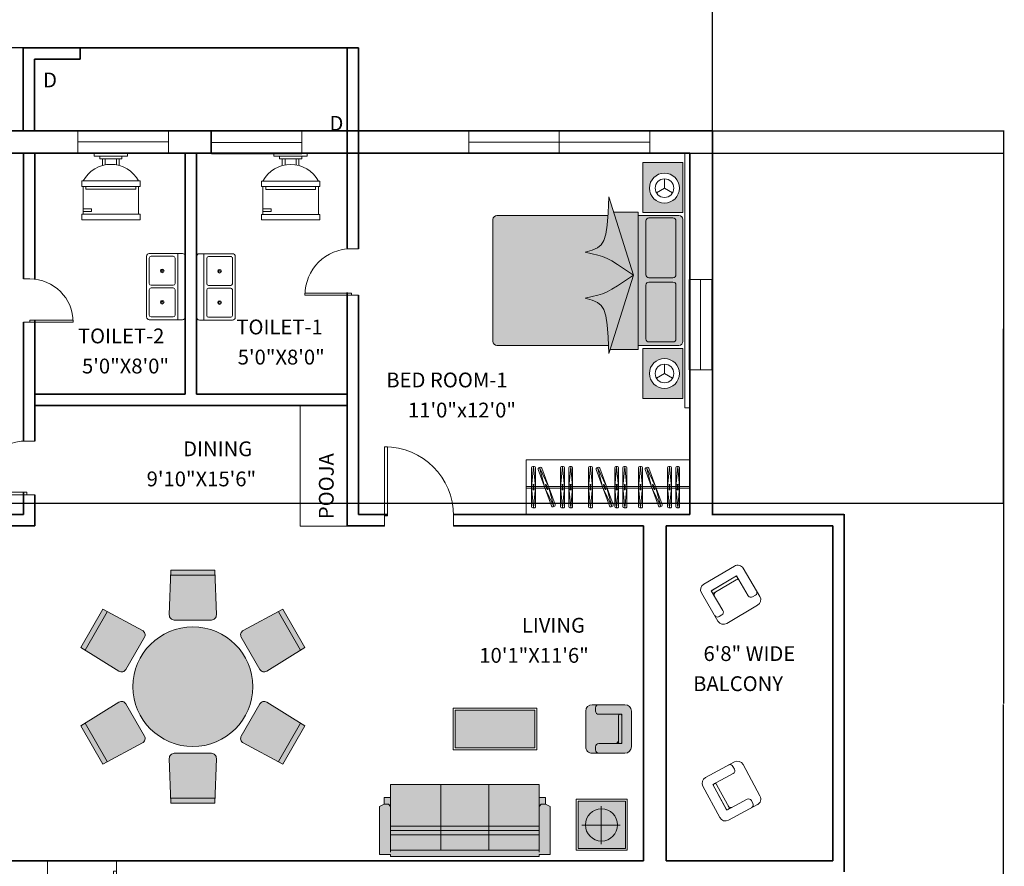
# Model space of a CAD drawing. Units: millimetres. Extents: x 27017497 to 27018854, y 7058029 to 7059154.
# Tile 90 of 91: x 27018462 to 27018854, y 7058297 to 7058634. Entities that reach past the tile are written whole.
import ezdxf

# ---------------------------------------------------------------- set-up
doc = ezdxf.new("R2010")
doc.units = ezdxf.units.MM
for name, color, linetype, lineweight in [('A-ANNO-DIMS', 2, 'Continuous', 18), ('A-ANNO-IDEN', 7, 'Continuous', 18), ('A-AREA-IDEN', 7, 'Continuous', 18), ('A-DOOR', 4, 'Continuous', 20), ('A-FLOR-CASE', 8, 'Continuous', 20), ('A-FLOR-FIXT', 9, 'Continuous', 18), ('A-FURN', 8, 'Continuous', 18), ('A-GLAZ', 4, 'Continuous', 18), ('A-WALL', 7, 'Continuous', 35)]:
    doc.layers.add(name, color=color, linetype=linetype, lineweight=lineweight)
doc.layers.add('A-FURN-PATT', color=177, linetype='Continuous', lineweight=13, true_color=0x293189)
doc.styles.get("Standard").update_dxf_attribs({"font": 'arial.ttf'})
doc.dimstyles.get("Standard").update_dxf_attribs({"dimtxt": 0.18, "dimasz": 0.18, "dimexe": 0.18, "dimexo": 0.0625, "dimgap": 0.09, "dimtad": 0, "dimtih": 1, "dimtoh": 1, "dimdec": 4, "dimzin": 0, "dimdsep": 46, "dimtxsty": 'Standard', "dimcen": 0.09, "dimadec": 0, "dimazin": 0, "dimtfac": 1, "dimtdec": 4, "dimtofl": 0, "dimtmove": 0, "dimatfit": 3, "dimfxl": 1, "dimtolj": 1, "dimtzin": 0, "dimarcsym": 0})

# ---------------------------------------------------------------- blocks, each defined once
blk = doc.blocks.new('CAMMAT')
for p, q in [((1.2731, 0), (-1.2731, 0)), ((1.2731, 0), (1.2731, -0.05)), ((-1.2731, 0), (-1.2731, -0.05)), ((1.2731, -0.05), (-1.2731, -0.05)), ((-1.18, -0.07), (-1.18, -0.47)), ((-1.18, -0.07), (-0.68, -0.07)), ((-0.68, -0.07), (-0.68, -0.47)), ((0.61, -0.07), (-0.61, -0.07)), ((0.68, -0.07), (0.68, -0.47)), ((0.68, -0.07), (1.18, -0.07)), ((1.18, -0.07), (1.18, -0.47)), ((-0.931, -0.2541), (-0.9775, -0.1737)), ((-0.65, -0.11), (-0.65, -0.5169)), ((-0.6152, -0.1695), (-0.6152, -0.4095)), ((-0.0465, -0.1395), (-0.5852, -0.1395)), ((-0.0165, -0.1695), (-0.0165, -0.4095)), ((0.0274, -0.1695), (0.0274, -0.4095)), ((0.5962, -0.1395), (0.0574, -0.1395)), ((0.6262, -0.1695), (0.6262, -0.4095)), ((0.65, -0.11), (0.65, -0.5169)), ((0.9242, -0.2541), (0.8777, -0.1737)), ((-0.931, -0.2541), (-0.9775, -0.3346)), ((-0.931, -0.2541), (-0.8381, -0.2541)), ((0.9242, -0.2541), (0.8777, -0.3346)), ((0.9242, -0.2541), (1.0171, -0.2541)), ((-1.18, -0.47), (-0.68, -0.47)), ((-0.0465, -0.4395), (-0.5852, -0.4395)), ((0.5962, -0.4395), (0.0574, -0.4395)), ((0.68, -0.47), (1.18, -0.47)), ((0.0535, -0.5623), (-0.7312, -0.8093)), ((-0.6904, -0.5169), (-0.6904, -0.8)), ((-0.6904, -0.5169), (0.6826, -0.5169)), ((0.0535, -0.5623), (0.8382, -0.8093)), ((0.6826, -0.5169), (0.6826, -0.7603)), ((-0.65, -0.8139), (-0.65, -1.93)), ((0.65, -0.8204), (0.65, -1.93)), ((0.61, -1.97), (-0.61, -1.97))]:
    blk.add_line(p, q)
for points in [[(-0.1761, -1.0476), (-0.161, -0.9772), (-0.1474, -0.921), (-0.1326, -0.8732), (-0.1139, -0.8282), (-0.0886, -0.7803), (-0.0541, -0.7238), (-0.0076, -0.653), (0.0535, -0.5623)], [(0.2832, -1.0476), (0.2681, -0.9772), (0.2545, -0.921), (0.2396, -0.8732), (0.2209, -0.8282), (0.1957, -0.7803), (0.1611, -0.7238), (0.1147, -0.653), (0.0535, -0.5623)], [(-0.7312, -0.8093), (-0.5683, -0.8185), (-0.4451, -0.828), (-0.3552, -0.8406), (-0.2919, -0.8591), (-0.2489, -0.8862), (-0.2196, -0.9248), (-0.1975, -0.9777), (-0.1761, -1.0476)], [(0.8382, -0.8093), (0.6753, -0.8185), (0.5522, -0.828), (0.4622, -0.8406), (0.399, -0.8591), (0.356, -0.8862), (0.3267, -0.9248), (0.3046, -0.9777), (0.2832, -1.0476)]]:
    blk.add_lwpolyline(points)
for centre, radius in [((-0.931, -0.2541), 0.15), ((-0.931, -0.2541), 0.0929), ((0.9242, -0.2541), 0.15), ((0.9242, -0.2541), 0.0929)]:
    blk.add_circle(centre, radius)
for centre, radius, start, end in [((-0.61, -0.11), 0.04, 90, 180), ((0.61, -0.11), 0.04, 0, 90), ((-0.5852, -0.1695), 0.03, 90, 180), ((-0.0465, -0.1695), 0.03, 360, 90), ((0.0574, -0.1695), 0.03, 90, 180), ((0.5962, -0.1695), 0.03, 360, 90), ((-0.5852, -0.4095), 0.03, 180, 270), ((-0.0465, -0.4095), 0.03, 270, 360), ((0.0574, -0.4095), 0.03, 180, 270), ((0.5962, -0.4095), 0.03, 270, 360), ((-0.61, -1.93), 0.04, 180, 270), ((0.61, -1.93), 0.04, 270, 360)]:
    blk.add_arc(centre, radius, start, end)
blk = doc.blocks.new('*U2')
for p, q in [((0, 0), (0, -6)), ((40, 0), (40, -6))]:
    blk.add_line(p, q)
blk.add_lwpolyline([(0, 0), (0, 40), (1.75, 40), (1.75, 0)], close=True)
blk.add_arc((0, 0), 40, 0, 90)
blk = doc.blocks.new('6 Person Round 01')
for points in [[(-235.8, 1886.7), (-220.8, 2335), (220.8, 2335), (235.8, 1886.7, -0.424007), (185.8, 1835), (-185.8, 1835, -0.424007)], [(-740.7, 1322.9), (-1121.5, 1560), (-900.7, 1942.5), (-504.9, 1731.3, -0.424007), (-485.2, 1662.2), (-671, 1340.3, -0.424007)], [(504.9, 1731.3), (900.7, 1942.5), (1121.5, 1560), (740.7, 1322.9, -0.424007), (671, 1340.3), (485.2, 1662.2, -0.424007)], [(-504.9, 603.7), (-900.7, 392.5), (-1121.5, 775), (-740.7, 1012.1, -0.424007), (-671, 994.7), (-485.2, 672.8, -0.424007)], [(740.7, 1012.1), (1121.5, 775), (900.7, 392.5), (504.9, 603.7, -0.424007), (485.2, 672.8), (671, 994.7, -0.424007)], [(235.8, 448.3), (220.8, 0), (-220.8, 0), (-235.8, 448.3, -0.424007), (-185.8, 500), (185.8, 500, -0.424007)]]:
    blk.add_lwpolyline(points, format="xyb", close=True)
for points in [[(222.5, 2285), (-222.5, 2285)], [(-856.5, 1918.9), (-1079, 1533.6)], [(1079, 1533.6), (856.5, 1918.9)], [(-1079, 801.4), (-856.5, 416.1)], [(856.5, 416.1), (1079, 801.4)], [(-222.5, 50), (222.5, 50)]]:
    blk.add_lwpolyline(points)
blk.add_circle((0, 1167.5), 600)
blk = doc.blocks.new('*U6')
for p, q in [((-10, 22), (-10, 12)), ((10, 12), (10, 22)), ((-10, 21), (-7, 21)), ((-7, 20), (-10, 20)), ((-7, 21), (-7, 20)), ((10.5, 12), (-10.5, 12)), ((-10.5, 10), (-10.5, 12)), ((9, 13), (-9, 13)), ((-9, 13), (-9, 12)), ((9, 12), (9, 13)), ((10.5, 12), (10.5, 10)), ((10.5, 10), (-10.5, 10)), ((-3, 4.4065), (-3, 2)), ((-2, 2), (-2, 4.1658)), ((2, 4.1658), (2, 2)), ((3, 2), (3, 4.4065)), ((4, 2), (-4, 2)), ((-4, 2), (-4, 1)), ((4, 1), (4, 2))]:
    blk.add_line(p, q)
for points in [[(10.5, 22), (10.5, 24), (-10.5, 24), (-10.5, 22)], [(6, 0), (6, 1), (-6, 1), (-6, 0)]]:
    blk.add_lwpolyline(points, close=True)
blk.add_arc((0, 15.3333), 11.3333, 208.0725, 331.9275)
blk = doc.blocks.new('Sink-double - 36 in top')
for p, q in [((-18, -4), (18, -4)), ((-0.75, -18.5), (-0.75, -6.5)), ((0.75, -6.5), (0.75, -18.5))]:
    blk.add_line(p, q)
for points in [[(-16.5, 0), (16.5, 0)], [(-18, -19.5), (-18, -1.5)], [(18, -1.5), (18, -19.5)], [(-16.5, -18.5), (-16.5, -6.5)], [(-15.5, -5.5), (-1.75, -5.5)], [(1.75, -5.5), (15.5, -5.5)], [(16.5, -6.5), (16.5, -18.5)], [(16.5, -21), (-16.5, -21)], [(-1.75, -19.5), (-15.5, -19.5)], [(15.5, -19.5), (1.75, -19.5)]]:
    blk.add_lwpolyline(points)
for centre, radius in [((-8.5, -12.5), 1), ((-8.5, -12.5), 0.5), ((8.5, -12.5), 1), ((8.5, -12.5), 0.5)]:
    blk.add_circle(centre, radius)
for centre, radius, start, end in [((-16.5, -1.5), 1.5, 90, 180), ((16.5, -1.5), 1.5, 0, 90), ((-15.5, -6.5), 1, 90, 180), ((-1.75, -6.5), 1, 0, 90), ((1.75, -6.5), 1, 90, 180), ((15.5, -6.5), 1, 0, 90), ((-16.5, -19.5), 1.5, 180, 270), ((-15.5, -18.5), 1, 180, 270), ((-1.75, -18.5), 1, 270, 0), ((1.75, -18.5), 1, 180, 270), ((15.5, -18.5), 1, 270, 0), ((16.5, -19.5), 1.5, 270, 0)]:
    blk.add_arc(centre, radius, start, end)
blk = doc.blocks.new('CHAIR-OCCASIONAL')
for p, q in [((3.87, 20.42), (0.09, 6.71)), ((19.6, 18.74), (7.02, 22.21)), ((4.13, 6.92), (7.23, 18.17)), ((5.25, 10.97), (7.23, 18.17)), ((5.25, 10.97), (7.1, 17.68)), ((8.33, 17.34), (5.63, 7.52)), ((16.06, 15.73), (7.23, 18.17)), ((7.23, 18.17), (16.06, 15.73)), ((7.23, 18.17), (16.06, 15.73)), ((7.73, 18.03), (7.97, 17.97)), ((7.73, 18.03), (7.97, 17.97)), ((17.64, 16.63), (17.98, 17.86)), ((17.64, 16.63), (17.98, 17.86)), ((17.6, 1.88), (21.39, 15.6)), ((12.96, 4.48), (4.13, 6.92)), ((4.87, 6.71), (4.63, 6.78)), ((5.63, 7.52), (5.5, 7.07)), ((1.88, 3.56), (14.46, 0.09)), ((13.86, 2.91), (13.52, 1.68))]:
    blk.add_line(p, q)
for centre, radius, start, end in [((6.34, 19.74), 2.56, 74.5879, 164.5879), ((7.59, 17.54), 0.512, 74.5879, 164.5879), ((7.84, 17.47), 0.512, 344.5879, 74.5879), ((9.36, 16.26), 1.28, 74.5879, 164.5879), ((16.4, 16.97), 1.28, 254.5879, 344.5879), ((16.4, 16.97), 1.28, 254.5879, 344.5879), ((16.74, 18.2), 1.28, 344.5879, 74.5879), ((16.74, 18.2), 1.28, 344.5879, 74.5879), ((18.92, 16.28), 2.56, 344.5879, 74.5879), ((2.56, 6.03), 2.56, 164.5879, 254.5879), ((4.76, 7.28), 0.512, 164.5879, 254.5879), ((5.01, 7.21), 0.512, 254.5879, 344.5879), ((12.62, 3.25), 1.28, 344.5879, 74.5879), ((12.28, 2.02), 1.28, 254.5879, 344.5879), ((15.14, 2.56), 2.56, 254.5879, 344.5879)]:
    blk.add_arc(centre, radius, start, end)
blk = doc.blocks.new('SOFA-LIVING-THREE-SEAT')
for p, q in [((63.53, 28.72), (4.35, 28.72)), ((4.35, 28.72), (4.35, 23.5)), ((24.37, 28.72), (24.37, 2.61)), ((43.51, 28.72), (43.51, 2.61)), ((63.53, 23.5), (63.53, 28.72)), ((1.74, 20.89), (0, 20.02)), ((0, 20.02), (0, 0.87)), ((4.35, 23.5), (1.74, 23.5)), ((1.74, 23.5), (1.74, 20.89)), ((1.74, 20.89), (3.48, 20.89)), ((3.48, 20.89), (4.35, 20.02)), ((4.35, 23.5), (4.35, 20.02)), ((4.35, 20.02), (4.35, 1.74)), ((63.53, 23.5), (63.53, 20.02)), ((66.14, 23.5), (63.53, 23.5)), ((64.4, 20.89), (63.53, 20.02)), ((63.53, 20.02), (63.53, 1.74)), ((66.14, 20.89), (64.4, 20.89)), ((66.14, 20.89), (66.14, 23.5)), ((67.88, 20.02), (66.14, 20.89)), ((67.88, 0.87), (67.88, 20.02)), ((63.53, 12.18), (4.35, 12.18)), ((63.53, 10.44), (4.35, 10.44)), ((63.53, 8.7), (4.35, 8.7)), ((0, 0.87), (4.35, 0.87)), ((4.35, 2.61), (63.53, 2.61)), ((4.35, 0.87), (4.35, 0)), ((4.35, 0), (63.53, 0)), ((63.53, 0), (63.53, 0.87)), ((63.53, 0.87), (67.88, 0.87))]:
    blk.add_line(p, q)
blk = doc.blocks.new('TABLE-END-LIVING')
for p, q in [((20.34, 20.34), (0, 20.34)), ((0, 20.34), (0, 0)), ((20.34, 0), (20.34, 20.34)), ((19.6, 19.6), (0.74, 19.6)), ((0.74, 19.6), (0.74, 0.74)), ((10.36, 2.37), (10.36, 17.54)), ((19.6, 0.74), (19.6, 19.6)), ((2.83, 10), (18.06, 10)), ((0, 0), (20.34, 0)), ((0.74, 0.74), (19.6, 0.74))]:
    blk.add_line(p, q)
blk.add_circle((10.28, 10.08), 6.4)
blk = doc.blocks.new('TABLE-COFFEE')
for p, q in [((33.35, 16.67), (0, 16.67)), ((0, 16.67), (0, 0)), ((32.51, 15.84), (0.83, 15.84)), ((0.83, 15.84), (0.83, 0.83)), ((32.51, 0.83), (32.51, 15.84)), ((33.35, 0), (33.35, 16.67)), ((0, 0), (33.35, 0)), ((0.83, 0.83), (32.51, 0.83))]:
    blk.add_line(p, q)
blk = doc.blocks.new('WARDROBE-HANGING-WALL-BACKED')
for p, q in [((0, 21.74), (65.21, 21.74)), ((0, 0), (0, 21.74)), ((65.21, 0), (65.21, 21.74)), ((4.86, 19.15), (4.08, 10.88)), ((4.08, 18.62), (4.08, 3.13)), ((5.18, 19.15), (4.55, 19.15)), ((4.86, 19.15), (5.64, 10.88)), ((5.64, 18.62), (5.64, 3.13)), ((8.14, 19.15), (7.35, 10.88)), ((7.35, 18.62), (7.35, 3.13)), ((8.45, 19.15), (7.82, 19.15)), ((8.14, 19.15), (8.92, 10.88)), ((8.92, 18.62), (8.92, 3.13)), ((16.33, 18.5), (11.03, 3.94)), ((17.8, 17.96), (12.5, 3.4)), ((17.25, 18.73), (13.68, 11.22)), ((17.25, 18.73), (15.15, 10.68)), ((17.54, 18.62), (16.95, 18.83)), ((19.66, 19.15), (18.88, 10.88)), ((18.88, 18.62), (18.88, 3.13)), ((19.98, 19.15), (19.35, 19.15)), ((19.66, 19.15), (20.45, 10.88)), ((20.45, 18.62), (20.45, 3.13)), ((25.9, 19.15), (25.12, 10.88)), ((25.12, 18.62), (25.12, 3.13)), ((26.21, 19.15), (25.59, 19.15)), ((25.9, 19.15), (26.68, 10.88)), ((26.68, 18.62), (26.68, 3.13)), ((29.17, 19.15), (28.39, 10.88)), ((28.39, 18.62), (28.39, 3.13)), ((29.49, 19.15), (28.86, 19.15)), ((29.17, 19.15), (29.96, 10.88)), ((29.96, 18.62), (29.96, 3.13)), ((35.87, 18.5), (30.57, 3.94)), ((37.34, 17.96), (32.04, 3.4)), ((36.78, 18.73), (33.22, 11.22)), ((36.78, 18.73), (34.69, 10.68)), ((37.08, 18.62), (36.49, 18.83)), ((39.59, 19.15), (38.81, 10.88)), ((38.81, 18.62), (38.81, 3.13)), ((39.9, 19.15), (39.28, 19.15)), ((39.59, 19.15), (40.37, 10.88)), ((40.37, 18.62), (40.37, 3.13)), ((47.49, 19.15), (46.71, 10.88)), ((46.71, 18.62), (46.71, 3.13)), ((47.81, 19.15), (47.18, 19.15)), ((47.49, 19.15), (48.28, 10.88)), ((48.28, 18.62), (48.28, 3.13)), ((50.77, 19.15), (49.98, 10.88)), ((49.98, 18.62), (49.98, 3.13)), ((51.08, 19.15), (50.45, 19.15)), ((50.77, 19.15), (51.55, 10.88)), ((51.55, 18.62), (51.55, 3.13)), ((58.96, 18.5), (53.66, 3.94)), ((60.43, 17.96), (55.13, 3.4)), ((59.88, 18.73), (56.31, 11.22)), ((59.88, 18.73), (57.78, 10.68)), ((60.17, 18.62), (59.58, 18.83)), ((62.29, 19.15), (61.51, 10.88)), ((61.51, 18.62), (61.51, 3.13)), ((62.61, 19.15), (61.98, 19.15)), ((62.29, 19.15), (63.08, 10.88)), ((63.08, 18.62), (63.08, 3.13)), ((4.71, 11.83), (4.71, 9.93)), ((4.92, 11.93), (4.8, 11.93)), ((5.02, 11.83), (5.02, 9.93)), ((7.98, 11.83), (7.98, 9.93)), ((8.2, 11.93), (8.07, 11.93)), ((8.29, 11.83), (8.29, 9.93)), ((14.59, 11.9), (13.94, 10.11)), ((14.89, 11.79), (14.24, 10)), ((14.84, 11.92), (14.72, 11.96)), ((19.51, 11.83), (19.51, 9.93)), ((19.73, 11.93), (19.6, 11.93)), ((19.82, 11.83), (19.82, 9.93)), ((25.74, 11.83), (25.74, 9.93)), ((25.96, 11.93), (25.84, 11.93)), ((26.06, 11.83), (26.06, 9.93)), ((29.02, 11.83), (29.02, 9.93)), ((29.24, 11.93), (29.11, 11.93)), ((29.33, 11.83), (29.33, 9.93)), ((34.13, 11.9), (33.48, 10.11)), ((34.42, 11.79), (33.77, 10)), ((34.37, 11.92), (34.25, 11.96)), ((39.43, 11.83), (39.43, 9.93)), ((39.65, 11.93), (39.53, 11.93)), ((39.75, 11.83), (39.75, 9.93)), ((47.34, 11.83), (47.34, 9.93)), ((47.56, 11.93), (47.43, 11.93)), ((47.65, 11.83), (47.65, 9.93)), ((50.61, 11.83), (50.61, 9.93)), ((50.83, 11.93), (50.7, 11.93)), ((50.92, 11.83), (50.92, 9.93)), ((57.22, 11.9), (56.57, 10.11)), ((57.52, 11.79), (56.87, 10)), ((57.47, 11.92), (57.35, 11.96)), ((62.14, 11.83), (62.14, 9.93)), ((62.36, 11.93), (62.23, 11.93)), ((62.45, 11.83), (62.45, 9.93)), ((0, 11.23), (65.21, 11.23)), ((0, 10.51), (65.21, 10.51)), ((4.86, 2.6), (4.08, 10.88)), ((4.92, 9.82), (4.8, 9.82)), ((4.86, 2.6), (5.64, 10.88)), ((8.14, 2.6), (7.35, 10.88)), ((8.2, 9.82), (8.07, 9.82)), ((8.14, 2.6), (8.92, 10.88)), ((11.59, 3.17), (13.68, 11.22)), ((11.59, 3.17), (15.15, 10.68)), ((14.11, 9.94), (14, 9.98)), ((19.66, 2.6), (18.88, 10.88)), ((19.73, 9.82), (19.6, 9.82)), ((19.66, 2.6), (20.45, 10.88)), ((25.9, 2.6), (25.12, 10.88)), ((25.96, 9.82), (25.84, 9.82)), ((25.9, 2.6), (26.68, 10.88)), ((29.17, 2.6), (28.39, 10.88)), ((29.24, 9.82), (29.11, 9.82)), ((29.17, 2.6), (29.96, 10.88)), ((31.12, 3.17), (33.22, 11.22)), ((31.12, 3.17), (34.69, 10.68)), ((33.65, 9.94), (33.53, 9.98)), ((39.59, 2.6), (38.81, 10.88)), ((39.65, 9.82), (39.53, 9.82)), ((39.59, 2.6), (40.37, 10.88)), ((47.49, 2.6), (46.71, 10.88)), ((47.56, 9.82), (47.43, 9.82)), ((47.49, 2.6), (48.28, 10.88)), ((50.77, 2.6), (49.98, 10.88)), ((50.83, 9.82), (50.7, 9.82)), ((50.77, 2.6), (51.55, 10.88)), ((54.22, 3.17), (56.31, 11.22)), ((54.22, 3.17), (57.78, 10.68)), ((56.74, 9.94), (56.63, 9.98)), ((62.29, 2.6), (61.51, 10.88)), ((62.36, 9.82), (62.23, 9.82)), ((62.29, 2.6), (63.08, 10.88)), ((5.18, 2.6), (4.55, 2.6)), ((8.45, 2.6), (7.82, 2.6)), ((11.88, 3.07), (11.29, 3.28)), ((19.98, 2.6), (19.35, 2.6)), ((26.21, 2.6), (25.59, 2.6)), ((29.49, 2.6), (28.86, 2.6)), ((31.42, 3.07), (30.83, 3.28)), ((39.9, 2.6), (39.28, 2.6)), ((47.81, 2.6), (47.18, 2.6)), ((51.08, 2.6), (50.45, 2.6)), ((54.51, 3.07), (53.92, 3.28)), ((62.61, 2.6), (61.98, 2.6))]:
    blk.add_line(p, q)
for centre, major_axis, start_param, end_param in [((4.55, 18.62), (0, 0.528), 0, 1.570796), ((5.18, 18.62), (0, 0.528), 4.712389, 6.283185), ((7.82, 18.62), (0, 0.528), 0, 1.570796), ((8.45, 18.62), (0, 0.528), 4.712389, 6.283185), ((16.77, 18.34), (0.181, 0.496), 0, 1.570796), ((17.36, 18.12), (0.181, 0.496), -1.570796, 0), ((19.35, 18.62), (0, 0.528), 0, 1.570796), ((19.98, 18.62), (0, 0.528), 4.712389, 6.283185), ((25.59, 18.62), (0, 0.528), 0, 1.570796), ((26.21, 18.62), (0, 0.528), 4.712389, 6.283185), ((28.86, 18.62), (0, 0.528), 0, 1.570796), ((29.49, 18.62), (0, 0.528), 4.712389, 6.283185), ((36.31, 18.34), (0.181, 0.496), 0, 1.570796), ((36.9, 18.12), (0.181, 0.496), -1.570796, 0), ((39.28, 18.62), (0, 0.528), 0, 1.570796), ((39.9, 18.62), (0, 0.528), 4.712389, 6.283185), ((47.18, 18.62), (0, 0.528), 0, 1.570796), ((47.81, 18.62), (0, 0.528), 4.712389, 6.283185), ((50.45, 18.62), (0, 0.528), 0, 1.570796), ((51.08, 18.62), (0, 0.528), 4.712389, 6.283185), ((59.4, 18.34), (0.181, 0.496), 0, 1.570796), ((59.99, 18.12), (0.181, 0.496), -1.570796, 0), ((61.98, 18.62), (0, 0.528), 0, 1.570796), ((62.61, 18.62), (0, 0.528), 4.712389, 6.283185), ((4.8, 11.83), (0, 0.106), 0, 1.570796), ((4.92, 11.83), (0, 0.106), -1.570796, 0), ((8.07, 11.83), (0, 0.106), 0, 1.570796), ((8.2, 11.83), (0, 0.106), -1.570796, 0), ((14.68, 11.86), (0.0361, 0.0993), 0, 1.570796), ((14.8, 11.82), (0.0361, 0.0993), 4.712389, 6.283185), ((19.6, 11.83), (0, 0.106), 0, 1.570796), ((19.73, 11.83), (0, 0.106), -1.570796, 0), ((25.84, 11.83), (0, 0.106), 0, 1.570796), ((25.96, 11.83), (0, 0.106), -1.570796, 0), ((29.11, 11.83), (0, 0.106), 0, 1.570796), ((29.24, 11.83), (0, 0.106), -1.570796, 0), ((34.22, 11.86), (0.0361, 0.0993), 0, 1.570796), ((34.34, 11.82), (0.0361, 0.0993), 4.712389, 6.283185), ((39.53, 11.83), (0, 0.106), 0, 1.570796), ((39.65, 11.83), (0, 0.106), -1.570796, 0), ((47.43, 11.83), (0, 0.106), 0, 1.570796), ((47.56, 11.83), (0, 0.106), -1.570796, 0), ((50.7, 11.83), (0, 0.106), 0, 1.570796), ((50.83, 11.83), (0, 0.106), -1.570796, 0), ((57.31, 11.86), (0.0361, 0.0993), 0, 1.570796), ((57.43, 11.82), (0.0361, 0.0993), 4.712389, 6.283185), ((62.23, 11.83), (0, 0.106), 0, 1.570796), ((62.36, 11.83), (0, 0.106), -1.570796, 0), ((4.8, 9.93), (0, 0.106), 1.570796, 3.141593), ((4.92, 9.93), (0, 0.106), 3.141593, 4.712389), ((8.07, 9.93), (0, 0.106), 1.570796, 3.141593), ((8.2, 9.93), (0, 0.106), 3.141593, 4.712389), ((14.03, 10.08), (0.0361, 0.0993), 1.570796, 3.141593), ((14.15, 10.03), (0.0361, 0.0993), 3.141593, 4.712389), ((19.6, 9.93), (0, 0.106), 1.570796, 3.141593), ((19.73, 9.93), (0, 0.106), 3.141593, 4.712389), ((25.84, 9.93), (0, 0.106), 1.570796, 3.141593), ((25.96, 9.93), (0, 0.106), 3.141593, 4.712389), ((29.11, 9.93), (0, 0.106), 1.570796, 3.141593), ((29.24, 9.93), (0, 0.106), 3.141593, 4.712389), ((33.57, 10.08), (0.0361, 0.0993), 1.570796, 3.141593), ((33.69, 10.03), (0.0361, 0.0993), 3.141593, 4.712389), ((39.53, 9.93), (0, 0.106), 1.570796, 3.141593), ((39.65, 9.93), (0, 0.106), 3.141593, 4.712389), ((47.43, 9.93), (0, 0.106), 1.570796, 3.141593), ((47.56, 9.93), (0, 0.106), 3.141593, 4.712389), ((50.7, 9.93), (0, 0.106), 1.570796, 3.141593), ((50.83, 9.93), (0, 0.106), 3.141593, 4.712389), ((56.66, 10.08), (0.0361, 0.0993), 1.570796, 3.141593), ((56.78, 10.03), (0.0361, 0.0993), 3.141593, 4.712389), ((62.23, 9.93), (0, 0.106), 1.570796, 3.141593), ((62.36, 9.93), (0, 0.106), 3.141593, 4.712389), ((11.47, 3.78), (0.181, 0.496), 1.570796, 3.141593), ((31.01, 3.78), (0.181, 0.496), 1.570796, 3.141593), ((54.1, 3.78), (0.181, 0.496), 1.570796, 3.141593), ((4.55, 3.13), (0, 0.528), 1.570796, 3.141593), ((5.18, 3.13), (0, 0.528), 3.141593, 4.712389), ((7.82, 3.13), (0, 0.528), 1.570796, 3.141593), ((8.45, 3.13), (0, 0.528), 3.141593, 4.712389), ((12.06, 3.56), (0.181, 0.496), 3.141593, 4.712389), ((19.35, 3.13), (0, 0.528), 1.570796, 3.141593), ((19.98, 3.13), (0, 0.528), 3.141593, 4.712389), ((25.59, 3.13), (0, 0.528), 1.570796, 3.141593), ((26.21, 3.13), (0, 0.528), 3.141593, 4.712389), ((28.86, 3.13), (0, 0.528), 1.570796, 3.141593), ((29.49, 3.13), (0, 0.528), 3.141593, 4.712389), ((31.6, 3.56), (0.181, 0.496), 3.141593, 4.712389), ((39.28, 3.13), (0, 0.528), 1.570796, 3.141593), ((39.9, 3.13), (0, 0.528), 3.141593, 4.712389), ((47.18, 3.13), (0, 0.528), 1.570796, 3.141593), ((47.81, 3.13), (0, 0.528), 3.141593, 4.712389), ((50.45, 3.13), (0, 0.528), 1.570796, 3.141593), ((51.08, 3.13), (0, 0.528), 3.141593, 4.712389), ((54.69, 3.56), (0.181, 0.496), 3.141593, 4.712389), ((61.98, 3.13), (0, 0.528), 1.570796, 3.141593), ((62.61, 3.13), (0, 0.528), 3.141593, 4.712389)]:
    blk.add_ellipse(centre, major_axis=major_axis, ratio=0.888892, start_param=start_param, end_param=end_param)
blk = doc.blocks.new('WINDOW-SINGLE-LIGHT')
blk.add_lwpolyline([(36, 4.5), (36, 0), (0, 0), (0, 9), (36, 9), (36, 4.5), (0, 4.5)])
blk = doc.blocks.new('*D48')
at = {"layer": 'A-ANNO-DIMS', "color": 0, "lineweight": -2, "transparency": 16777216}
for p, q in [((27018463.5, 7058622.91), (27017497.54, 7058622.91)), ((27017497.72, 7058622.73), (27017497.72, 7058357.75)), ((27017497.72, 7058092.41), (27017497.72, 7058357.39)), ((27018555.13, 7058092.23), (27017497.54, 7058092.23))]:
    blk.add_line(p, q, dxfattribs=at)
at = {"layer": 'A-ANNO-DIMS', "color": 0, "transparency": 16777216}
for points in [[(27017497.69, 7058622.73), (27017497.75, 7058622.73), (27017497.72, 7058622.91)], [(27017497.69, 7058092.41), (27017497.75, 7058092.41), (27017497.72, 7058092.23)]]:
    blk.add_solid(points, dxfattribs=at)
at = {"layer": 'Defpoints', "color": 0, "transparency": 16777216}
for p in [(27018463.56, 7058622.91), (27017497.72, 7058092.23), (27018555.19, 7058092.23)]:
    blk.add_point(p, dxfattribs=at)
at = {"layer": 'A-ANNO-DIMS', "color": 0, "transparency": 16777216, "insert": (27017497.72, 7058357.57), "char_height": 0.18, "attachment_point": 5}
blk.add_mtext('\\A1;530.7', dxfattribs=at)
blk = doc.blocks.new('*D50')
at = {"layer": 'A-ANNO-DIMS', "color": 0, "lineweight": -2, "transparency": 16777216}
for p, q in [((27018223.67, 7058580.91), (27018854.24, 7058580.91)), ((27018854.06, 7058580.73), (27018854.06, 7058511.34)), ((27018854.06, 7058441.59), (27018854.06, 7058510.98)), ((27018223.67, 7058441.41), (27018854.24, 7058441.41))]:
    blk.add_line(p, q, dxfattribs=at)
at = {"layer": 'A-ANNO-DIMS', "color": 0, "transparency": 16777216}
for points in [[(27018854.03, 7058580.73), (27018854.09, 7058580.73), (27018854.06, 7058580.91)], [(27018854.03, 7058441.59), (27018854.09, 7058441.59), (27018854.06, 7058441.41)]]:
    blk.add_solid(points, dxfattribs=at)
at = {"layer": 'Defpoints', "color": 0, "transparency": 16777216}
for p in [(27018223.61, 7058580.91), (27018223.61, 7058441.41), (27018854.06, 7058441.41)]:
    blk.add_point(p, dxfattribs=at)
at = {"layer": 'A-ANNO-DIMS', "color": 0, "transparency": 16777216, "insert": (27018854.06, 7058511.16), "char_height": 0.18, "attachment_point": 5}
blk.add_mtext('\\A1;139.5', dxfattribs=at)
blk = doc.blocks.new('*D52')
at = {"layer": 'A-ANNO-DIMS', "color": 0, "lineweight": -2, "transparency": 16777216}
for p, q in [((27018310.61, 7058589.97), (27018310.61, 7058686.54)), ((27018310.79, 7058686.36), (27018523.96, 7058686.36)), ((27018737.93, 7058686.36), (27018524.75, 7058686.36)), ((27018738.11, 7058589.97), (27018738.11, 7058686.54))]:
    blk.add_line(p, q, dxfattribs=at)
at = {"layer": 'A-ANNO-DIMS', "color": 0, "transparency": 16777216}
for points in [[(27018310.79, 7058686.39), (27018310.79, 7058686.33), (27018310.61, 7058686.36)], [(27018737.93, 7058686.39), (27018737.93, 7058686.33), (27018738.11, 7058686.36)]]:
    blk.add_solid(points, dxfattribs=at)
at = {"layer": 'Defpoints', "color": 0, "transparency": 16777216}
for p in [(27018738.11, 7058686.36), (27018310.61, 7058589.91), (27018738.11, 7058589.91)]:
    blk.add_point(p, dxfattribs=at)
at = {"layer": 'A-ANNO-DIMS', "color": 0, "transparency": 16777216, "insert": (27018524.36, 7058686.36), "char_height": 0.18, "attachment_point": 5}
blk.add_mtext('\\A1;427.5', dxfattribs=at)
blk = doc.blocks.new('*D53')
at = {"layer": 'A-ANNO-DIMS', "color": 0, "lineweight": -2, "transparency": 16777216}
for p, q in [((27018738.17, 7058589.91), (27018854.24, 7058589.91)), ((27018854.06, 7058589.73), (27018854.06, 7058361.59)), ((27018854.06, 7058133.09), (27018854.06, 7058361.23)), ((27018738.17, 7058132.91), (27018854.24, 7058132.91))]:
    blk.add_line(p, q, dxfattribs=at)
at = {"layer": 'A-ANNO-DIMS', "color": 0, "transparency": 16777216}
for points in [[(27018854.03, 7058589.73), (27018854.09, 7058589.73), (27018854.06, 7058589.91)], [(27018854.03, 7058133.09), (27018854.09, 7058133.09), (27018854.06, 7058132.91)]]:
    blk.add_solid(points, dxfattribs=at)
at = {"layer": 'Defpoints', "color": 0, "transparency": 16777216}
for p in [(27018738.11, 7058589.91), (27018854.06, 7058589.91), (27018738.11, 7058132.91)]:
    blk.add_point(p, dxfattribs=at)
at = {"layer": 'A-ANNO-DIMS', "color": 0, "transparency": 16777216, "insert": (27018854.06, 7058361.41), "char_height": 0.18, "attachment_point": 5}
blk.add_mtext('\\A1;457', dxfattribs=at)

msp = doc.modelspace()

# ---------------------------------------------------------------- hatches: boundary and pattern name
at = {"layer": 'A-FURN-PATT'}
h = msp.add_hatch(color=256, dxfattribs=at)
h.dxf.hatch_style = 1
h.paths.add_polyline_path([(27018698.026, 7058538), (27018696.118, 7058539.006), (27018694.326, 7058539.751), (27018692.423, 7058540.341), (27018690.182, 7058540.884), (27018687.377, 7058541.486), (27018690.163, 7058542.338), (27018692.269, 7058543.218), (27018693.807, 7058544.385), (27018694.888, 7058546.099), (27018695.624, 7058548.617), (27018696.126, 7058552.199), (27018696.426, 7058556.096), (27018652.233, 7058556.096, 0.4142136), (27018650.639, 7058554.502), (27018650.639, 7058505.91, 0.4142136), (27018652.233, 7058504.317), (27018696.688, 7058504.317), (27018696.504, 7058507.572), (27018696.126, 7058512.478), (27018695.624, 7058516.06), (27018694.888, 7058518.579), (27018693.807, 7058520.292), (27018692.269, 7058521.459), (27018690.163, 7058522.339), (27018687.377, 7058523.191), (27018690.182, 7058523.794), (27018692.423, 7058524.336), (27018694.326, 7058524.926), (27018696.118, 7058525.671), (27018698.026, 7058526.677), (27018700.276, 7058528.052), (27018703.094, 7058529.904), (27018706.708, 7058532.339), (27018703.094, 7058534.773), (27018700.276, 7058536.625)])
h.paths.add_polyline_path([(27018696.871, 7058563.593), (27018696.504, 7058557.105), (27018696.126, 7058552.199), (27018695.624, 7058548.617), (27018694.888, 7058546.099), (27018693.807, 7058544.385), (27018692.269, 7058543.218), (27018690.163, 7058542.338), (27018687.377, 7058541.486), (27018690.182, 7058540.884), (27018692.423, 7058540.341), (27018694.326, 7058539.751), (27018696.118, 7058539.006), (27018698.026, 7058538), (27018700.276, 7058536.625), (27018703.094, 7058534.773), (27018706.708, 7058532.339)])
h.paths.add_polyline_path([(27018706.708, 7058532.339), (27018703.094, 7058529.904), (27018700.276, 7058528.052), (27018698.026, 7058526.677), (27018696.118, 7058525.671), (27018694.326, 7058524.926), (27018692.423, 7058524.336), (27018690.182, 7058523.794), (27018687.377, 7058523.191), (27018690.163, 7058522.339), (27018692.269, 7058521.459), (27018693.807, 7058520.292), (27018694.888, 7058518.579), (27018695.624, 7058516.06), (27018696.126, 7058512.478), (27018696.504, 7058507.572), (27018696.871, 7058501.084)])
h.paths.add_polyline_path([(27018708.515, 7058557.393), (27018698.822, 7058557.393), (27018706.708, 7058532.339), (27018697.382, 7058502.708), (27018708.515, 7058502.708)])
h.paths.add_polyline_path([(27018726.316, 7058554.502, 0.4142136), (27018724.723, 7058556.096), (27018708.515, 7058556.096), (27018708.515, 7058504.317), (27018724.723, 7058504.317, 0.4142136), (27018726.316, 7058505.91)])
h.paths.add_polyline_path([(27018712.794, 7058529.551), (27018722.353, 7058529.551, -0.4142136), (27018723.548, 7058528.356), (27018723.548, 7058506.896, -0.4142136), (27018722.353, 7058505.701), (27018712.794, 7058505.701, -0.4142136), (27018711.599, 7058506.896), (27018711.599, 7058528.356, -0.4142136)], flags=16)
h.paths.add_polyline_path([(27018711.599, 7058532.493), (27018711.599, 7058553.952, -0.4142136), (27018712.794, 7058555.147), (27018722.353, 7058555.147, -0.4142136), (27018723.548, 7058553.952), (27018723.548, 7058532.493, -0.4142136), (27018722.353, 7058531.298), (27018712.794, 7058531.298, -0.4142136)], flags=0)
h.paths.add_polyline_path([(27018726.316, 7058577.205), (27018710.384, 7058577.205), (27018710.384, 7058557.29), (27018726.316, 7058557.29)])
h.paths.add_polyline_path([(27018724.958, 7058567.015, -1), (27018713.009, 7058567.015, -1)], flags=16)
h.paths.add_polyline_path([(27018722.683, 7058567.015, -1), (27018715.284, 7058567.015, -1)], flags=0)
h.paths.add_polyline_path([(27018726.316, 7058503.122), (27018710.384, 7058503.122), (27018710.384, 7058483.207), (27018726.316, 7058483.207)])
h.paths.add_polyline_path([(27018713.009, 7058493.123, -1), (27018724.958, 7058493.123, -1)], flags=16)
h.paths.add_polyline_path([(27018715.284, 7058493.123, -1), (27018722.683, 7058493.123, -1)], flags=0)
h.paths.add_polyline_path([(27018723.548, 7058528.356, 0.4142136), (27018722.353, 7058529.551), (27018712.794, 7058529.551, 0.4142136), (27018711.599, 7058528.356), (27018711.599, 7058506.896, 0.4142136), (27018712.794, 7058505.701), (27018722.353, 7058505.701, 0.4142136), (27018723.548, 7058506.896)], flags=16)
h.paths.add_polyline_path([(27018723.548, 7058553.952, 0.4142136), (27018722.353, 7058555.147), (27018712.794, 7058555.147, 0.4142136), (27018711.599, 7058553.952), (27018711.599, 7058532.493, 0.4142136), (27018712.794, 7058531.298), (27018722.353, 7058531.298, 0.4142136), (27018723.548, 7058532.493)], flags=16)
h = msp.add_hatch(color=256, dxfattribs=at)
h.dxf.hatch_style = 1
h.paths.add_polyline_path([(27018723.548, 7058553.952, 0.4142136), (27018722.353, 7058555.147), (27018712.794, 7058555.147, 0.4142136), (27018711.599, 7058553.952), (27018711.599, 7058532.493, 0.4142136), (27018712.794, 7058531.298), (27018722.353, 7058531.298, 0.4142136), (27018723.548, 7058532.493)])
h = msp.add_hatch(color=256, dxfattribs=at)
h.dxf.hatch_style = 1
h.paths.add_polyline_path([(27018507.232, 7058368.275, 1), (27018554.972, 7058368.275, 1)])
h.paths.add_polyline_path([(27018565.178, 7058398.17), (27018551.19, 7058390.704, 0.4240071), (27018550.404, 7058387.955), (27018557.796, 7058375.151, 0.4240071), (27018560.57, 7058374.457), (27018574.03, 7058382.838)])
h.paths.add_polyline_path([(27018574.03, 7058353.712), (27018560.57, 7058362.093, 0.4240071), (27018557.796, 7058361.399), (27018550.404, 7058348.596, 0.4240071), (27018551.19, 7058345.846), (27018565.178, 7058338.38)])
h.paths.add_polyline_path([(27018540.482, 7058339.664, 0.4240071), (27018538.494, 7058341.72), (27018523.71, 7058341.72, 0.4240071), (27018521.722, 7058339.664), (27018522.25, 7058323.817), (27018539.954, 7058323.817)], flags=17)
h.paths.add_polyline_path([(27018511.8, 7058348.596), (27018504.408, 7058361.399, 0.4240071), (27018501.634, 7058362.093), (27018488.174, 7058353.712), (27018497.026, 7058338.38), (27018511.014, 7058345.846, 0.4240071)])
h.paths.add_polyline_path([(27018511.8, 7058387.955, 0.4240071), (27018511.014, 7058390.704), (27018497.026, 7058398.17), (27018488.174, 7058382.838), (27018501.634, 7058374.457, 0.4240071), (27018504.408, 7058375.151)])
h.paths.add_polyline_path([(27018539.954, 7058412.733), (27018522.25, 7058412.733), (27018521.722, 7058396.886, 0.4240071), (27018523.71, 7058394.831), (27018538.494, 7058394.831, 0.4240071), (27018540.482, 7058396.886)])
h.paths.add_polyline_path([(27018566.934, 7058399.107), (27018565.178, 7058398.17), (27018574.03, 7058382.838), (27018575.719, 7058383.89)])
h.paths.add_polyline_path([(27018575.719, 7058352.66), (27018574.03, 7058353.712), (27018565.178, 7058338.38), (27018566.934, 7058337.443)])
h.paths.add_polyline_path([(27018540.482, 7058339.664, 0.4240071), (27018538.494, 7058341.72), (27018523.71, 7058341.72, 0.4240071), (27018521.722, 7058339.664), (27018522.25, 7058323.817), (27018522.316, 7058321.828), (27018539.887, 7058321.828)])
h.paths.add_polyline_path([(27018488.174, 7058353.712), (27018486.484, 7058352.66), (27018495.27, 7058337.443), (27018497.026, 7058338.38)])
h.paths.add_polyline_path([(27018497.026, 7058398.17), (27018495.27, 7058399.107), (27018486.484, 7058383.89), (27018488.174, 7058382.838)])
h.paths.add_polyline_path([(27018539.887, 7058414.723), (27018522.316, 7058414.723), (27018522.25, 7058412.733), (27018539.954, 7058412.733)])
h = msp.add_hatch(color=256, dxfattribs=at)
h.dxf.hatch_style = 1
h.paths.add_polyline_path([(27018667.323, 7058358.933), (27018635.645, 7058358.933), (27018635.645, 7058343.928), (27018667.323, 7058343.928)])
h.paths.add_polyline_path([(27018703.409, 7058322.68), (27018684.545, 7058322.68), (27018684.545, 7058303.816), (27018703.409, 7058303.816)])
h.paths.add_polyline_path([(27018700.269, 7058313.072), (27018693.785, 7058313.072), (27018693.785, 7058306.75, 0.4142112)], flags=16)
h.paths.add_polyline_path([(27018703.232, 7058361.098), (27018692.792, 7058361.098, 0.4142136), (27018691.513, 7058359.819), (27018691.513, 7058358.539, 0.4142136), (27018692.792, 7058357.26), (27018701.952, 7058357.26), (27018701.952, 7058345.59), (27018692.792, 7058345.59, 0.4142136), (27018691.513, 7058344.31), (27018691.513, 7058343.031, 0.4142136), (27018692.792, 7058341.751), (27018703.232, 7058341.751, 0.4142136), (27018705.791, 7058344.31), (27018705.791, 7058358.539, 0.4142136)])
h.paths.add_polyline_path([(27018700.673, 7058356.283), (27018700.673, 7058356.748, -0.4142136), (27018701.184, 7058357.26), (27018692.792, 7058357.26, -0.4142136), (27018691.513, 7058358.539), (27018691.513, 7058359.819, -0.4142136), (27018692.792, 7058361.098), (27018690.183, 7058361.098, 0.4142136), (27018687.624, 7058358.539), (27018687.624, 7058344.31, 0.4142136), (27018690.183, 7058341.751), (27018692.792, 7058341.751, -0.4142136), (27018691.513, 7058343.031), (27018691.513, 7058344.31, -0.4142136), (27018692.792, 7058345.59), (27018699.393, 7058345.59, 0.4142136), (27018700.673, 7058346.869)])
h.paths.add_polyline_path([(27018701.952, 7058353.053), (27018701.952, 7058356.748, 0.4142136), (27018701.44, 7058357.26), (27018701.184, 7058357.26, 0.4142136), (27018700.673, 7058356.748), (27018700.673, 7058356.283), (27018700.673, 7058346.101, 0.4142136), (27018701.184, 7058345.59), (27018701.44, 7058345.59, 0.4142136), (27018701.952, 7058346.101)], flags=17)
h = msp.add_hatch(color=256, dxfattribs=at)
h.dxf.hatch_style = 1
h.paths.add_polyline_path([(27018540.482, 7058339.664, 0.4240071), (27018538.494, 7058341.72), (27018523.71, 7058341.72, 0.4240071), (27018521.722, 7058339.664), (27018522.25, 7058323.817), (27018539.954, 7058323.817)])
h = msp.add_hatch(color=256, dxfattribs=at)
h.dxf.hatch_style = 1
h.paths.add_polyline_path([(27018629.877, 7058329.264), (27018609.86, 7058329.264), (27018609.86, 7058324.042), (27018609.86, 7058320.561), (27018609.86, 7058312.728), (27018629.877, 7058312.728)])
h.paths.add_polyline_path([(27018649.023, 7058329.264), (27018629.877, 7058329.264), (27018629.877, 7058312.728), (27018649.023, 7058312.728)])
h.paths.add_polyline_path([(27018669.04, 7058324.042), (27018669.04, 7058329.264), (27018649.023, 7058329.264), (27018649.023, 7058312.728), (27018669.04, 7058312.728), (27018669.04, 7058320.561)])
h.paths.add_polyline_path([(27018669.04, 7058309.247), (27018649.023, 7058309.247), (27018649.023, 7058303.155), (27018669.04, 7058303.155)], flags=17)
h.paths.add_polyline_path([(27018649.023, 7058309.247), (27018629.877, 7058309.247), (27018629.877, 7058303.155), (27018649.023, 7058303.155)], flags=17)
h.paths.add_polyline_path([(27018629.877, 7058309.247), (27018609.86, 7058309.247), (27018609.86, 7058303.155), (27018629.877, 7058303.155)], flags=17)
h.paths.add_polyline_path([(27018629.877, 7058312.728), (27018609.86, 7058312.728), (27018609.86, 7058310.988), (27018629.877, 7058310.988)], flags=17)
h.paths.add_polyline_path([(27018629.877, 7058310.988), (27018609.86, 7058310.988), (27018609.86, 7058309.247), (27018629.877, 7058309.247)], flags=17)
h.paths.add_polyline_path([(27018649.023, 7058312.728), (27018629.877, 7058312.728), (27018629.877, 7058310.988), (27018649.023, 7058310.988)], flags=17)
h.paths.add_polyline_path([(27018669.04, 7058312.728), (27018649.023, 7058312.728), (27018649.023, 7058310.988), (27018669.04, 7058310.988)], flags=17)
h.paths.add_polyline_path([(27018669.04, 7058310.988), (27018649.023, 7058310.988), (27018649.023, 7058309.247), (27018669.04, 7058309.247)], flags=17)
h.paths.add_polyline_path([(27018649.023, 7058310.988), (27018629.877, 7058310.988), (27018629.877, 7058309.247), (27018649.023, 7058309.247)], flags=17)
h.paths.add_polyline_path([(27018609.86, 7058320.561), (27018608.99, 7058321.431), (27018607.249, 7058321.431), (27018605.509, 7058320.561), (27018605.509, 7058301.415), (27018609.86, 7058301.415), (27018609.86, 7058300.544), (27018669.04, 7058300.544), (27018669.04, 7058301.415), (27018673.392, 7058301.415), (27018673.392, 7058320.561), (27018671.651, 7058321.431), (27018669.91, 7058321.431), (27018669.04, 7058320.561), (27018669.04, 7058303.155), (27018609.86, 7058303.155)])
h.paths.add_polyline_path([(27018609.86, 7058324.042), (27018607.249, 7058324.042), (27018607.249, 7058321.431), (27018608.99, 7058321.431), (27018609.86, 7058320.561)])
h.paths.add_polyline_path([(27018671.651, 7058324.042), (27018669.04, 7058324.042), (27018669.04, 7058320.561), (27018669.91, 7058321.431), (27018671.651, 7058321.431)])
h = msp.add_hatch(color=256, dxfattribs=at)
h.dxf.hatch_style = 1
h.paths.add_polyline_path([(27018700.269, 7058313.072), (27018693.785, 7058313.072), (27018693.785, 7058306.75, 0.4142112)])

# ---------------------------------------------------------------- linework, layer by layer
at = {"layer": 'A-FLOR-CASE'}
for p, q in [((27018573.903, 7058432.276), (27018573.903, 7058480.412)), ((27018592.89, 7058432.276), (27018573.903, 7058432.276))]:
    msp.add_line(p, q, dxfattribs=at)
at = {"layer": 'A-GLAZ'}
msp.add_lwpolyline([(27018538.322, 7058589.881), (27018521.36, 7058589.881), (27018521.36, 7058580.963), (27018538.322, 7058580.963)], close=True, dxfattribs=at)
at = {"layer": 'A-WALL'}
for p, q in [((27018463.561, 7058589.912), (27018463.561, 7058622.912)), ((27018463.561, 7058622.912), (27018486.239, 7058622.912)), ((27018486.239, 7058622.912), (27018597.106, 7058622.912)), ((27018486.239, 7058618.412), (27018486.239, 7058622.912)), ((27018592.606, 7058622.912), (27018592.606, 7058543.053)), ((27018597.106, 7058622.912), (27018597.106, 7058542.877)), ((27018468.061, 7058589.912), (27018468.061, 7058618.412)), ((27018468.061, 7058618.412), (27018486.239, 7058618.412)), ((27018738.106, 7058589.912), (27018310.606, 7058589.912)), ((27018738.106, 7058589.912), (27018738.106, 7058437.098)), ((27018729.106, 7058580.912), (27018319.606, 7058580.912)), ((27018463.606, 7058580.912), (27018463.606, 7058530.804)), ((27018468.106, 7058580.912), (27018468.106, 7058530.724)), ((27018528.106, 7058580.912), (27018528.106, 7058484.912)), ((27018532.606, 7058580.912), (27018532.606, 7058484.912)), ((27018729.106, 7058580.912), (27018729.106, 7058436.912)), ((27018592.606, 7058525.375), (27018592.606, 7058432.412)), ((27018597.106, 7058524.331), (27018597.106, 7058436.912)), ((27018463.606, 7058513.597), (27018463.606, 7058466.164)), ((27018468.106, 7058514.376), (27018468.106, 7058466.205)), ((27018528.106, 7058484.912), (27018468.106, 7058484.912)), ((27018592.606, 7058484.912), (27018532.606, 7058484.912)), ((27018532.606, 7058480.412), (27018468.106, 7058480.412)), ((27018592.606, 7058480.412), (27018532.606, 7058480.412)), ((27018463.606, 7058445.749), (27018463.606, 7058436.912)), ((27018468.106, 7058444.814), (27018468.106, 7058432.412)), ((27018463.606, 7058436.912), (27018319.606, 7058436.912)), ((27018608.687, 7058436.912), (27018597.106, 7058436.912)), ((27018729.106, 7058436.912), (27018634.961, 7058436.912)), ((27018790.39, 7058436.905), (27018737.89, 7058436.905)), ((27018790.606, 7058437.098), (27018790.606, 7058294.412)), ((27018468.106, 7058432.412), (27018319.606, 7058432.412)), ((27018607.484, 7058432.412), (27018592.606, 7058432.412)), ((27018710.606, 7058432.412), (27018634.966, 7058432.412)), ((27018710.606, 7058432.412), (27018710.606, 7058298.912)), ((27018719.606, 7058432.412), (27018719.606, 7058298.912)), ((27018786.106, 7058432.412), (27018719.606, 7058432.412)), ((27018729.106, 7058432.412), (27018719.606, 7058432.412)), ((27018786.106, 7058432.412), (27018786.106, 7058298.912)), ((27018545.106, 7058298.912), (27018319.606, 7058298.912)), ((27018592.992, 7058298.912), (27018545.106, 7058298.912)), ((27018608.106, 7058298.912), (27018592.992, 7058298.912)), ((27018710.606, 7058298.912), (27018608.106, 7058298.912)), ((27018786.106, 7058298.912), (27018719.606, 7058298.912))]:
    msp.add_line(p, q, dxfattribs=at)

# ---------------------------------------------------------------- block references
at = {"layer": 'A-DOOR'}
for p, xscale, yscale, zscale, rotation in [((27018594.324, 7058524.331), 0.4636703714562217, 0.4636703714562217, 0.4636703714562217, 90.00000000000003), ((27018466.179, 7058513.597), -0.4301822298564029, 0.4301822298564029, 0.4301822298564029, 270), ((27018464.924, 7058444.814), 0.5347783892510444, 0.5347783892510444, 0.5347783892510444, 90.00000000000003), ((27018500.714, 7058294.79), 0.6870473523349573, 0.6870473523349573, 0.6870473523349573, 180)]:
    msp.add_blockref('*U2', p, dxfattribs=dict(at, xscale=xscale, yscale=yscale, zscale=zscale, rotation=rotation))
at = {"layer": 'A-DOOR', "xscale": 0.6870473523349573, "yscale": 0.6870473523349573, "zscale": 0.6870473523349573}
msp.add_blockref('*U2', (27018607.484, 7058436.382), dxfattribs=at)
at = {"layer": 'A-FLOR-CASE', "extrusion": (0, 0, -1), "zscale": -1}
msp.add_blockref('WARDROBE-HANGING-WALL-BACKED', (-27018729.107, 7058436.905), dxfattribs=at)
at = {"layer": 'A-FLOR-FIXT'}
for name, p, xscale, yscale, zscale, rotation in [('*U6', (27018498.447, 7058580.908), -1.105119395603938, 1.105119395603938, 1.105119395603938, 180), ('*U6', (27018570.058, 7058580.878), -1.105119395603938, 1.105119395603938, 1.105119395603938, 180), ('Sink-double - 36 in top', (27018528.071, 7058527.759), -0.7340308267416257, 0.7340308267416257, 0.7340308267416257, 270), ('Sink-double - 36 in top', (27018532.591, 7058527.641), 0.7340308267416257, 0.7340308267416257, 0.7340308267416257, 90.00000000000003)]:
    msp.add_blockref(name, p, dxfattribs=dict(at, xscale=xscale, yscale=yscale, zscale=zscale, rotation=rotation))
at = {"layer": 'A-FURN', "xscale": -39.82996475819422, "yscale": 39.82996475819422, "zscale": 39.82996475819422, "rotation": 270}
msp.add_blockref('CAMMAT', (27018729.104, 7058530.206), dxfattribs=at)
at = {"layer": 'A-FURN', "extrusion": (0, 0, -1), "zscale": -1}
for p, rotation in [((-27018753.32, 7058418.198), 254.9680663077895), ((-27018732.703, 7058335.139), 167.1010863143652)]:
    msp.add_blockref('CHAIR-OCCASIONAL', p, dxfattribs=dict(at, rotation=rotation))
at = {"layer": 'A-FURN', "xscale": -0.0397836222497725, "yscale": 0.0397836222497725, "zscale": 0.0397836222497725}
msp.add_blockref('6 Person Round 01', (27018531.102, 7058321.828), dxfattribs=at)
at = {"layer": 'A-FURN'}
for name, p, rotation in [('CHAIR-OCCASIONAL', (27018704.097, 7058365.028), 195.4121391531662), ('TABLE-COFFEE', (27018668.157, 7058359.767), 180)]:
    msp.add_blockref(name, p, dxfattribs=dict(at, rotation=rotation))
at = {"layer": 'A-FURN', "extrusion": (0, 0, -1), "zscale": -1}
for name, p in [('SOFA-LIVING-THREE-SEAT', (-27018673.392, 7058300.544)), ('TABLE-END-LIVING', (-27018704.149, 7058303.076))]:
    msp.add_blockref(name, p, dxfattribs=at)
at = {"layer": 'A-GLAZ', "extrusion": (0, 0, -1), "zscale": -1}
for p in [(-27018521.347, 7058580.903), (-27018574.48, 7058580.67), (-27018677.091, 7058580.889), (-27018713.086, 7058580.886)]:
    msp.add_blockref('WINDOW-SINGLE-LIGHT', p, dxfattribs=at)
at = {"layer": 'A-GLAZ', "extrusion": (0, 0, -1), "zscale": -1, "rotation": 270}
msp.add_blockref('WINDOW-SINGLE-LIGHT', (-27018737.811, 7058530.539), dxfattribs=at)

# ---------------------------------------------------------------- texts
at = {"layer": 'A-ANNO-DIMS'}
for s, height, p in [('5\'0"X8\'0"', 5.9118, (27018548.973, 7058496.704)), ('5\'0"X8\'0"', 5.9118, (27018486.95, 7058493.134)), ('11\'0"x12\'0"', 5.91176, (27018616.81, 7058475.579)), ('9\'10"X15\'6"', 5.91176, (27018512.69, 7058448.139)), ('10\'1"X11\'6"', 5.91176, (27018645.216, 7058377.8)), ('6\'8" WIDE', 5.9118, (27018734.524, 7058378.509))]:
    msp.add_text(s, height=height, dxfattribs=at).set_placement(p)
at = {"layer": 'A-ANNO-IDEN'}
for p in [(27018471.445, 7058607.171), (27018585.529, 7058589.912)]:
    msp.add_text('D', height=5.912, rotation=360, dxfattribs=at).set_placement(p)
at = {"layer": 'A-AREA-IDEN'}
for s, p in [('TOILET-1', (27018548.432, 7058508.701)), ('TOILET-2', (27018485.328, 7058505.131)), ('BED ROOM-1', (27018608.162, 7058487.577)), ('DINING', (27018527.239, 7058460.137)), ('LIVING', (27018662.18, 7058389.798)), ('BALCONY', (27018730.396, 7058366.512))]:
    msp.add_text(s, height=5.9118, dxfattribs=at).set_placement(p)
msp.add_text('POOJA', height=5.9118, rotation=90, dxfattribs=at).set_placement((27018587.209, 7058435.06))

# ---------------------------------------------------------------- dimensions: what is measured, and where the dimension line sits
at = {"layer": 'A-ANNO-DIMS'}
dim = msp.add_linear_dim(base=(27018738.106, 7058686.362), p1=(27018310.606, 7058589.912), p2=(27018738.106, 7058589.912), dimstyle='Standard', override={"dimdec": 1, "dimlfac": 1, "dimrnd": 0, "dimzin": 0, "dimdsep": 46, "dimlunit": 2}, dxfattribs=at)
dim.commit()
dim.dimension.update_dxf_attribs({"geometry": '*D52', "text_midpoint": (27018524.356, 7058686.362)})
for base, p1, p2, override, picture, middle in [((27017497.716, 7058092.23), (27018463.561, 7058622.912), (27018555.192, 7058092.23), {"dimdec": 1, "dimlfac": 1, "dimrnd": 0, "dimzin": 0, "dimdsep": 46, "dimlunit": 2}, '*D48', (27017497.716, 7058357.571)), ((27018854.056, 7058589.912), (27018738.106, 7058132.912), (27018738.106, 7058589.912), {"dimdec": 0, "dimlfac": 1, "dimrnd": 0, "dimzin": 0, "dimdsep": 46, "dimlunit": 2}, '*D53', (27018854.056, 7058361.412)), ((27018854.056, 7058441.412), (27018223.606, 7058580.912), (27018223.606, 7058441.412), {"dimdec": 1, "dimlfac": 1, "dimrnd": 0, "dimzin": 0, "dimdsep": 46, "dimlunit": 2}, '*D50', (27018854.056, 7058511.162))]:
    dim = msp.add_linear_dim(base=base, p1=p1, p2=p2, angle=90, dimstyle='Standard', override=override, dxfattribs=at)
    dim.commit()
    dim.dimension.update_dxf_attribs({"geometry": picture, "text_midpoint": middle})

doc.saveas('drawing.dxf')
